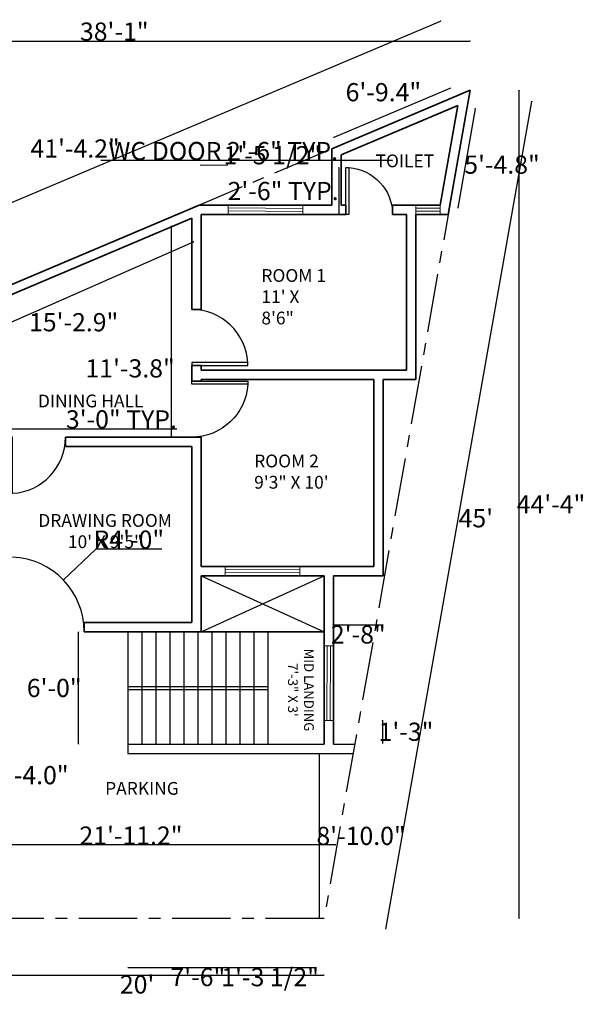
# Model space of a CAD drawing. Units: inches. Extents: x -496 to 183, y 146 to 778.
# Tile 2 of 2: x -180 to 183, y 146 to 778. Entities that reach past the tile are written whole.
import ezdxf

# ---------------------------------------------------------------- set-up
doc = ezdxf.new("R2010")
doc.units = ezdxf.units.IN
doc.header["$MEASUREMENT"] = 0
doc.linetypes.add('CENTER', pattern=[2, 1.25, -0.25, 0.25, -0.25])
for name, color, linetype, lineweight in [('A-ANNO-DIMS', 5, 'Continuous', 18), ('A-AREA-IDEN', 7, 'Continuous', 18), ('A-DOOR', 30, 'Continuous', 25), ('A-FLOR-STRS', 7, 'Continuous', 25), ('A-GLAZ', 2, 'Continuous', 18), ('A-WALL', 7, 'Continuous', 35), ('C-PROP', 3, 'CENTER', 25)]:
    doc.layers.add(name, color=color, linetype=linetype, lineweight=lineweight)
doc.styles.get("Standard").update_dxf_attribs({"font": 'arial.ttf'})
doc.dimstyles.get("Standard").update_dxf_attribs({"dimtxt": 11.68, "dimasz": 0.18, "dimexe": 0.18, "dimexo": 0.0625, "dimgap": 0.09, "dimtad": 2, "dimtih": 1, "dimtoh": 1, "dimdec": 1, "dimzin": 0, "dimdsep": 46, "dimlunit": 3, "dimtxsty": 'Standard', "dimblk": 'OPEN30', "dimcen": 0.09, "dimse1": 1, "dimse2": 1, "dimadec": 0, "dimazin": 0, "dimtfac": 1, "dimtdec": 1, "dimtofl": 0, "dimtmove": 0, "dimatfit": 3, "dimfxl": 1, "dimtolj": 1, "dimtzin": 0, "dimarcsym": 0})

# ---------------------------------------------------------------- blocks, each defined once
blk = doc.blocks.new('_Open30')
at = {"color": 0, "linetype": 'ByBlock', "lineweight": -2}
for p, q in [((-1, 0.27), (0, 0)), ((0, 0), (-1, -0.27)), ((0, 0), (-1, 0))]:
    blk.add_line(p, q, dxfattribs=at)
blk = doc.blocks.new('*D3')
at = {"layer": 'A-ANNO-DIMS', "color": 0, "lineweight": -2, "ltscale": 5, "transparency": 16777216}
blk.add_line((-224.62, 164.47), (15.02, 164.47), dxfattribs=at)
at = {"layer": 'Defpoints', "color": 0, "ltscale": 5, "transparency": 16777216}
for p in [(-224.8, 200.81), (15.2, 200.81), (15.2, 164.47)]:
    blk.add_point(p, dxfattribs=at)
at = {"layer": 'A-ANNO-DIMS', "color": 0, "lineweight": -2, "ltscale": 5, "transparency": 16777216, "xscale": 0.18, "yscale": 0.18, "zscale": 0.18, "rotation": 180}
blk.add_blockref('_Open30', (-224.8, 164.47), dxfattribs=at)
at = {"layer": 'A-ANNO-DIMS', "color": 0, "lineweight": -2, "ltscale": 5, "transparency": 16777216, "xscale": 0.18, "yscale": 0.18, "zscale": 0.18}
blk.add_blockref('_Open30', (15.2, 164.47), dxfattribs=at)
at = {"layer": 'A-ANNO-DIMS', "color": 0, "ltscale": 5, "transparency": 16777216, "insert": (-104.8, 158.42), "char_height": 11.68, "attachment_point": 5}
blk.add_mtext("\\A1;20'", dxfattribs=at)
blk = doc.blocks.new('*D4')
at = {"layer": 'A-ANNO-DIMS', "color": 0, "lineweight": -2, "ltscale": 5, "transparency": 16777216}
blk.add_line((54.9, 194), (148.6, 725.44), dxfattribs=at)
at = {"layer": 'Defpoints', "color": 0, "ltscale": 5, "transparency": 16777216}
for p in [(108.97, 732.61), (148.63, 725.62), (15.2, 200.81)]:
    blk.add_point(p, dxfattribs=at)
at = {"layer": 'A-ANNO-DIMS', "color": 0, "lineweight": -2, "ltscale": 5, "transparency": 16777216, "xscale": 0.18, "yscale": 0.18, "zscale": 0.18}
for p, rotation in [((148.63, 725.62), 80), ((54.86, 193.82), 260)]:
    blk.add_blockref('_Open30', p, dxfattribs=dict(at, rotation=rotation))
at = {"layer": 'A-ANNO-DIMS', "color": 0, "ltscale": 5, "transparency": 16777216, "insert": (112.71, 457.79), "char_height": 11.68, "attachment_point": 5}
blk.add_mtext("\\A1;45'", dxfattribs=at)
blk = doc.blocks.new('*D6')
at = {"layer": 'A-ANNO-DIMS', "color": 0, "lineweight": -2, "ltscale": 5, "transparency": 16777216}
blk.add_line((-366.62, 583.72), (89.94, 777.08), dxfattribs=at)
at = {"layer": 'Defpoints', "color": 0, "ltscale": 5, "transparency": 16777216}
for p in [(90.11, 777.15), (108.97, 732.61), (-347.92, 539.1)]:
    blk.add_point(p, dxfattribs=at)
at = {"layer": 'A-ANNO-DIMS', "color": 0, "lineweight": -2, "ltscale": 5, "transparency": 16777216, "xscale": 0.18, "yscale": 0.18, "zscale": 0.18}
for p, rotation in [((90.11, 777.15), 22.95381137769926), ((-366.79, 583.64), 202.9538113776993)]:
    blk.add_blockref('_Open30', p, dxfattribs=dict(at, rotation=rotation))
at = {"layer": 'A-ANNO-DIMS', "color": 0, "ltscale": 5, "transparency": 16777216, "insert": (-144.61, 695.21), "char_height": 11.68, "attachment_point": 5}
blk.add_mtext('\\A1;41\'-4.2"', dxfattribs=at)
blk = doc.blocks.new('*D7')
at = {"layer": 'A-ANNO-DIMS', "color": 0, "lineweight": -2, "ltscale": 5, "transparency": 16777216}
blk.add_line((-235.59, 561.64), (-68.58, 635.31), dxfattribs=at)
at = {"layer": 'Defpoints', "color": 0, "ltscale": 5, "transparency": 16777216}
for p in [(-69.77, 638.45), (-68.41, 635.38), (-237.11, 564.64)]:
    blk.add_point(p, dxfattribs=at)
at = {"layer": 'A-ANNO-DIMS', "color": 0, "lineweight": -2, "ltscale": 5, "transparency": 16777216, "xscale": 0.18, "yscale": 0.18, "zscale": 0.18}
for p, rotation in [((-68.41, 635.38), 23.80147962325558), ((-235.75, 561.57), 203.8014796232556)]:
    blk.add_blockref('_Open30', p, dxfattribs=dict(at, rotation=rotation))
at = {"layer": 'A-ANNO-DIMS', "color": 0, "ltscale": 5, "transparency": 16777216, "insert": (-145.55, 583.66), "char_height": 11.68, "attachment_point": 5}
blk.add_mtext('\\A1;15\'-2.9"', dxfattribs=at)
blk = doc.blocks.new('*D8')
at = {"layer": 'A-ANNO-DIMS', "color": 0, "lineweight": -2, "ltscale": 5, "transparency": 16777216}
blk.add_line((-82.89, 645.46), (-82.89, 509.99), dxfattribs=at)
at = {"layer": 'Defpoints', "color": 0, "ltscale": 5, "transparency": 16777216}
for p in [(-80.99, 645.64), (-82.89, 509.81), (-80.99, 509.81)]:
    blk.add_point(p, dxfattribs=at)
at = {"layer": 'A-ANNO-DIMS', "color": 0, "lineweight": -2, "ltscale": 5, "transparency": 16777216, "xscale": 0.18, "yscale": 0.18, "zscale": 0.18}
for p, rotation in [((-82.89, 645.64), 90), ((-82.89, 509.81), 270)]:
    blk.add_blockref('_Open30', p, dxfattribs=dict(at, rotation=rotation))
at = {"layer": 'A-ANNO-DIMS', "color": 0, "ltscale": 5, "transparency": 16777216, "insert": (-109.3, 554.01), "char_height": 11.68, "attachment_point": 5}
blk.add_mtext('\\A1;11\'-3.8"', dxfattribs=at)
blk = doc.blocks.new('*D9')
at = {"layer": 'A-ANNO-DIMS', "color": 0, "lineweight": -2, "ltscale": 5, "transparency": 16777216}
blk.add_line((112.33, 720.62), (101.13, 657.13), dxfattribs=at)
at = {"layer": 'Defpoints', "color": 0, "ltscale": 5, "transparency": 16777216}
for p in [(101.15, 722.78), (89.89, 658.93), (101.1, 656.96)]:
    blk.add_point(p, dxfattribs=at)
at = {"layer": 'A-ANNO-DIMS', "color": 0, "lineweight": -2, "ltscale": 5, "transparency": 16777216, "xscale": 0.18, "yscale": 0.18, "zscale": 0.18}
for p, rotation in [((112.36, 720.8), 79.99999999999996), ((101.1, 656.96), 260)]:
    blk.add_blockref('_Open30', p, dxfattribs=dict(at, rotation=rotation))
at = {"layer": 'A-ANNO-DIMS', "color": 0, "ltscale": 5, "transparency": 16777216, "insert": (129.51, 684.86), "char_height": 11.68, "attachment_point": 5}
blk.add_mtext('\\A1;5\'-4.8"', dxfattribs=at)
blk = doc.blocks.new('*D10')
at = {"layer": 'A-ANNO-DIMS', "color": 0, "lineweight": -2, "ltscale": 5, "transparency": 16777216}
blk.add_line((21.63, 702.39), (96.21, 733.98), dxfattribs=at)
at = {"layer": 'Defpoints', "color": 0, "ltscale": 5, "transparency": 16777216}
for p in [(96.37, 734.05), (101.15, 722.78), (26.23, 691.05)]:
    blk.add_point(p, dxfattribs=at)
at = {"layer": 'A-ANNO-DIMS', "color": 0, "lineweight": -2, "ltscale": 5, "transparency": 16777216, "xscale": 0.18, "yscale": 0.18, "zscale": 0.18}
for p, rotation in [((96.37, 734.05), 22.95381137769932), ((21.46, 702.32), 202.9538113776993)]:
    blk.add_blockref('_Open30', p, dxfattribs=dict(at, rotation=rotation))
at = {"layer": 'A-ANNO-DIMS', "color": 0, "ltscale": 5, "transparency": 16777216, "insert": (53.33, 731.38), "char_height": 11.68, "attachment_point": 5}
blk.add_mtext('\\A1;6\'-9.4"', dxfattribs=at)
blk = doc.blocks.new('*D11')
at = {"layer": 'A-ANNO-DIMS', "color": 0, "lineweight": -2, "ltscale": 5, "transparency": 16777216}
blk.add_line((12.02, 306.63), (12.02, 200.99), dxfattribs=at)
at = {"layer": 'Defpoints', "color": 0, "ltscale": 5, "transparency": 16777216}
for p in [(4.85, 306.81), (4.85, 200.81), (12.02, 200.81)]:
    blk.add_point(p, dxfattribs=at)
at = {"layer": 'A-ANNO-DIMS', "color": 0, "lineweight": -2, "ltscale": 5, "transparency": 16777216, "xscale": 0.18, "yscale": 0.18, "zscale": 0.18}
for p, rotation in [((12.02, 306.81), 90), ((12.02, 200.81), 270)]:
    blk.add_blockref('_Open30', p, dxfattribs=dict(at, rotation=rotation))
at = {"layer": 'A-ANNO-DIMS', "color": 0, "ltscale": 5, "transparency": 16777216, "insert": (38.99, 253.81), "char_height": 11.68, "attachment_point": 5}
blk.add_mtext('\\A1;8\'-10.0"', dxfattribs=at)
blk = doc.blocks.new('*D12')
at = {"layer": 'A-ANNO-DIMS', "color": 0, "lineweight": -2, "ltscale": 5, "transparency": 16777216}
blk.add_line((22.65, 248.06), (-240.18, 248.06), dxfattribs=at)
at = {"layer": 'Defpoints', "color": 0, "ltscale": 5, "transparency": 16777216}
for p in [(-240.36, 248.06), (-240.36, 243.58), (22.83, 244.08)]:
    blk.add_point(p, dxfattribs=at)
at = {"layer": 'A-ANNO-DIMS', "color": 0, "lineweight": -2, "ltscale": 5, "transparency": 16777216, "xscale": 0.18, "yscale": 0.18, "zscale": 0.18, "rotation": 180}
blk.add_blockref('_Open30', (-240.36, 248.06), dxfattribs=at)
at = {"layer": 'A-ANNO-DIMS', "color": 0, "lineweight": -2, "ltscale": 5, "transparency": 16777216, "xscale": 0.18, "yscale": 0.18, "zscale": 0.18}
blk.add_blockref('_Open30', (22.83, 248.06), dxfattribs=at)
at = {"layer": 'A-ANNO-DIMS', "color": 0, "ltscale": 5, "transparency": 16777216, "insert": (-108.76, 254.01), "char_height": 11.68, "attachment_point": 5}
blk.add_mtext('\\A1;21\'-11.2"', dxfattribs=at)
blk = doc.blocks.new('*D13')
at = {"layer": 'A-ANNO-DIMS', "color": 0, "lineweight": -2, "ltscale": 5, "transparency": 16777216}
blk.add_line((-203.87, 200.99), (-203.87, 384.63), dxfattribs=at)
at = {"layer": 'Defpoints', "color": 0, "ltscale": 5, "transparency": 16777216}
for p in [(-208.53, 384.81), (-203.87, 384.81), (-208.53, 200.81)]:
    blk.add_point(p, dxfattribs=at)
at = {"layer": 'A-ANNO-DIMS', "color": 0, "lineweight": -2, "ltscale": 5, "transparency": 16777216, "xscale": 0.18, "yscale": 0.18, "zscale": 0.18}
for p, rotation in [((-203.87, 384.81), 90), ((-203.87, 200.81), 270)]:
    blk.add_blockref('_Open30', p, dxfattribs=dict(at, rotation=rotation))
at = {"layer": 'A-ANNO-DIMS', "color": 0, "ltscale": 5, "transparency": 16777216, "insert": (-177.47, 292.81), "char_height": 11.68, "attachment_point": 5}
blk.add_mtext('\\A1;15\'-4.0"', dxfattribs=at)
blk = doc.blocks.new('DOOR-SWING-36IN')
at = {"ltscale": 5}
for p, q in [((0, 0), (0, -36)), ((2, 0), (0, 0)), ((2, -36), (2, 0)), ((0, -36), (2, -36))]:
    blk.add_line(p, q, dxfattribs=at)
blk.add_arc((-0.06, 0), 36.06, 273.27315, 0, dxfattribs=at)
blk = doc.blocks.new('DOOR-SWING-30IN')
at = {"ltscale": 5}
for p, q in [((0, 0), (-30, 0)), ((-30, 0), (-30, -2)), ((0, -2), (0, 0)), ((-30, -2), (0, -2))]:
    blk.add_line(p, q, dxfattribs=at)
blk.add_arc((0, 0.07), 30.07, 183.94987, 270, dxfattribs=at)
blk = doc.blocks.new('WIN-48IN')
at = {"ltscale": 5}
for p, q in [((0, 0), (-0.22, -48)), ((0, 0), (6, -0.03)), ((6, -0.03), (5.78, -48.03)), ((-0.22, -48), (5.78, -48.03))]:
    blk.add_line(p, q, dxfattribs=at)
for p, q in [((1.78, -48.01), (2, -0.01)), ((3.78, -48.02), (4, -0.02))]:
    blk.add_line(p, q)
blk = doc.blocks.new('WIN-SMALL-WC')
at = {"ltscale": 5}
for p, q in [((-15.66, -6), (-15.66, 0)), ((-15.66, 0), (0, 0)), ((0, 0), (0, -6)), ((-15.66, -2), (0, -2)), ((0, -4), (-15.66, -4)), ((0, -6), (-15.66, -6))]:
    blk.add_line(p, q, dxfattribs=at)
blk = doc.blocks.new('*D21')
at = {"layer": 'A-ANNO-DIMS', "color": 0, "lineweight": -2, "ltscale": 5, "transparency": 16777216}
for p, q in [((-186.59, 515.21), (-150.95, 515.21)), ((-150.77, 515.21), (-79.22, 515.21))]:
    blk.add_line(p, q, dxfattribs=at)
at = {"layer": 'Defpoints', "color": 0, "ltscale": 5, "transparency": 16777216}
for p in [(-150.77, 515.21), (-186.77, 509.81), (-150.77, 509.81)]:
    blk.add_point(p, dxfattribs=at)
at = {"layer": 'A-ANNO-DIMS', "color": 0, "lineweight": -2, "ltscale": 5, "transparency": 16777216, "xscale": 0.18, "yscale": 0.18, "zscale": 0.18, "rotation": 180}
blk.add_blockref('_Open30', (-186.77, 515.21), dxfattribs=at)
at = {"layer": 'A-ANNO-DIMS', "color": 0, "lineweight": -2, "ltscale": 5, "transparency": 16777216, "xscale": 0.18, "yscale": 0.18, "zscale": 0.18}
blk.add_blockref('_Open30', (-150.77, 515.21), dxfattribs=at)
at = {"layer": 'A-ANNO-DIMS', "color": 0, "ltscale": 5, "transparency": 16777216, "insert": (-114.9, 521.27), "char_height": 11.68, "attachment_point": 5}
blk.add_mtext('\\A1;3\'-0" TYP.', dxfattribs=at)
blk = doc.blocks.new('*D22')
at = {"layer": 'A-ANNO-DIMS', "color": 0, "lineweight": -2, "ltscale": 5, "transparency": 16777216}
for p, q in [((29.23, 687.43), (-128, 687.43)), ((59.05, 687.43), (29.41, 687.43))]:
    blk.add_line(p, q, dxfattribs=at)
at = {"layer": 'Defpoints', "color": 0, "ltscale": 5, "transparency": 16777216}
for p in [(29.23, 687.43), (29.23, 682.93), (59.23, 682.93)]:
    blk.add_point(p, dxfattribs=at)
at = {"layer": 'A-ANNO-DIMS', "color": 0, "lineweight": -2, "ltscale": 5, "transparency": 16777216, "xscale": 0.18, "yscale": 0.18, "zscale": 0.18}
for p, rotation in [((29.23, 687.43), 179.9999999999994), ((59.23, 687.43), 359.9999999999994)]:
    blk.add_blockref('_Open30', p, dxfattribs=dict(at, rotation=rotation))
at = {"layer": 'A-ANNO-DIMS', "color": 0, "ltscale": 5, "transparency": 16777216, "insert": (-49.47, 693.57), "char_height": 11.68, "attachment_point": 5}
blk.add_mtext('\\A1;WC DOOR 2\'-6" TYP.', dxfattribs=at)
blk = doc.blocks.new('*D23')
at = {"layer": 'A-ANNO-DIMS', "color": 0, "lineweight": -2, "ltscale": 5, "transparency": 16777216}
blk.add_line((24.73, 682.75), (24.73, 653.11), dxfattribs=at)
at = {"layer": 'Defpoints', "color": 0, "ltscale": 5, "transparency": 16777216}
for p in [(29.23, 682.93), (24.73, 652.93), (29.23, 652.93)]:
    blk.add_point(p, dxfattribs=at)
at = {"layer": 'A-ANNO-DIMS', "color": 0, "lineweight": -2, "ltscale": 5, "transparency": 16777216, "xscale": 0.18, "yscale": 0.18, "zscale": 0.18}
for p, rotation in [((24.73, 682.93), 90), ((24.73, 652.93), 270)]:
    blk.add_blockref('_Open30', p, dxfattribs=dict(at, rotation=rotation))
at = {"layer": 'A-ANNO-DIMS', "color": 0, "ltscale": 5, "transparency": 16777216, "insert": (-11.05, 667.93), "char_height": 11.68, "attachment_point": 5}
blk.add_mtext('\\A1;2\'-6" TYP.', dxfattribs=at)
blk = doc.blocks.new('*D28')
at = {"layer": 'A-ANNO-DIMS', "color": 0, "lineweight": -2, "ltscale": 5, "transparency": 16777216}
blk.add_line((-347.74, 764.21), (108.79, 764.21), dxfattribs=at)
at = {"layer": 'Defpoints', "color": 0, "ltscale": 5, "transparency": 16777216}
for p in [(108.97, 764.21), (108.97, 732.61), (-347.92, 539.1)]:
    blk.add_point(p, dxfattribs=at)
at = {"layer": 'A-ANNO-DIMS', "color": 0, "lineweight": -2, "ltscale": 5, "transparency": 16777216, "xscale": 0.18, "yscale": 0.18, "zscale": 0.18, "rotation": 180}
blk.add_blockref('_Open30', (-347.92, 764.21), dxfattribs=at)
at = {"layer": 'A-ANNO-DIMS', "color": 0, "lineweight": -2, "ltscale": 5, "transparency": 16777216, "xscale": 0.18, "yscale": 0.18, "zscale": 0.18}
blk.add_blockref('_Open30', (108.97, 764.21), dxfattribs=at)
at = {"layer": 'A-ANNO-DIMS', "color": 0, "ltscale": 5, "transparency": 16777216, "insert": (-119.47, 770.27), "char_height": 11.68, "attachment_point": 5}
blk.add_mtext('\\A1;38\'-1"', dxfattribs=at)
blk = doc.blocks.new('*D29')
at = {"layer": 'A-ANNO-DIMS', "color": 0, "lineweight": -2, "ltscale": 5, "transparency": 16777216}
blk.add_line((140.57, 200.99), (140.57, 732.43), dxfattribs=at)
at = {"layer": 'Defpoints', "color": 0, "ltscale": 5, "transparency": 16777216}
for p in [(108.97, 732.61), (140.57, 732.61), (15.2, 200.81)]:
    blk.add_point(p, dxfattribs=at)
at = {"layer": 'A-ANNO-DIMS', "color": 0, "lineweight": -2, "ltscale": 5, "transparency": 16777216, "xscale": 0.18, "yscale": 0.18, "zscale": 0.18}
for p, rotation in [((140.57, 732.61), 90), ((140.57, 200.81), 270)]:
    blk.add_blockref('_Open30', p, dxfattribs=dict(at, rotation=rotation))
at = {"layer": 'A-ANNO-DIMS', "color": 0, "ltscale": 5, "transparency": 16777216, "insert": (160.96, 466.71), "char_height": 11.68, "attachment_point": 5}
blk.add_mtext('\\A1;44\'-4"', dxfattribs=at)
blk = doc.blocks.new('*D30')
at = {"layer": 'A-ANNO-DIMS', "color": 0, "lineweight": -2, "ltscale": 5, "transparency": 16777216}
blk.add_line((-110.62, 169.21), (-20.98, 169.21), dxfattribs=at)
at = {"layer": 'Defpoints', "color": 0, "ltscale": 5, "transparency": 16777216}
for p in [(-110.8, 312.81), (-20.8, 312.81), (-20.8, 169.21)]:
    blk.add_point(p, dxfattribs=at)
at = {"layer": 'A-ANNO-DIMS', "color": 0, "lineweight": -2, "ltscale": 5, "transparency": 16777216, "xscale": 0.18, "yscale": 0.18, "zscale": 0.18, "rotation": 180}
blk.add_blockref('_Open30', (-110.8, 169.21), dxfattribs=at)
at = {"layer": 'A-ANNO-DIMS', "color": 0, "lineweight": -2, "ltscale": 5, "transparency": 16777216, "xscale": 0.18, "yscale": 0.18, "zscale": 0.18}
blk.add_blockref('_Open30', (-20.8, 169.21), dxfattribs=at)
at = {"layer": 'A-ANNO-DIMS', "color": 0, "ltscale": 5, "transparency": 16777216, "insert": (-65.8, 163.16), "char_height": 11.68, "attachment_point": 5}
blk.add_mtext('\\A1;7\'-6"', dxfattribs=at)
blk = doc.blocks.new('*D33')
at = {"layer": 'A-ANNO-DIMS', "color": 0, "lineweight": -2, "ltscale": 5, "transparency": 16777216}
for p, q in [((-63.59, 169.21), (-48.43, 169.21)), ((-48.25, 169.21), (9.27, 169.21))]:
    blk.add_line(p, q, dxfattribs=at)
at = {"layer": 'Defpoints', "color": 0, "ltscale": 5, "transparency": 16777216}
for p in [(-63.77, 426.81), (-48.25, 426.92), (-48.25, 169.21)]:
    blk.add_point(p, dxfattribs=at)
at = {"layer": 'A-ANNO-DIMS', "color": 0, "lineweight": -2, "ltscale": 5, "transparency": 16777216, "xscale": 0.18, "yscale": 0.18, "zscale": 0.18, "rotation": 180}
blk.add_blockref('_Open30', (-63.77, 169.21), dxfattribs=at)
at = {"layer": 'A-ANNO-DIMS', "color": 0, "lineweight": -2, "ltscale": 5, "transparency": 16777216, "xscale": 0.18, "yscale": 0.18, "zscale": 0.18}
blk.add_blockref('_Open30', (-48.25, 169.21), dxfattribs=at)
at = {"layer": 'A-ANNO-DIMS', "color": 0, "ltscale": 5, "transparency": 16777216, "insert": (-19.4, 163.08), "char_height": 11.68, "attachment_point": 5}
blk.add_mtext('\\A1;1\'-3 1/2"', dxfattribs=at)
blk = doc.blocks.new('*D34')
at = {"layer": 'A-ANNO-DIMS', "color": 0, "lineweight": -2, "ltscale": 5, "transparency": 16777216}
for p, q in [((-63.98, 684.53), (-47, 684.74)), ((-46.82, 684.75), (-46.64, 684.75))]:
    blk.add_line(p, q, dxfattribs=at)
at = {"layer": 'Defpoints', "color": 0, "ltscale": 5, "transparency": 16777216}
for p in [(-46.82, 684.75), (-63.77, 652.93), (-46.43, 653.15)]:
    blk.add_point(p, dxfattribs=at)
at = {"layer": 'A-ANNO-DIMS', "color": 0, "lineweight": -2, "ltscale": 5, "transparency": 16777216, "xscale": 0.18, "yscale": 0.18, "zscale": 0.18}
for p, rotation in [((-64.16, 684.53), 180.7141226270407), ((-46.82, 684.75), 0.7141226270407911)]:
    blk.add_blockref('_Open30', p, dxfattribs=dict(at, rotation=rotation))
at = {"layer": 'A-ANNO-DIMS', "color": 0, "ltscale": 5, "transparency": 16777216, "insert": (-17.97, 690.88), "char_height": 11.68, "attachment_point": 5}
blk.add_mtext('\\A1;1\'-5 1/2"', dxfattribs=at)
blk = doc.blocks.new('*D36')
at = {"layer": 'A-ANNO-DIMS', "color": 0, "lineweight": -2, "ltscale": 5, "transparency": 16777216}
blk.add_line((53.05, 389.21), (21.38, 389.21), dxfattribs=at)
at = {"layer": 'Defpoints', "color": 0, "ltscale": 5, "transparency": 16777216}
for p in [(21.2, 420.81), (53.23, 420.81), (21.2, 389.21)]:
    blk.add_point(p, dxfattribs=at)
at = {"layer": 'A-ANNO-DIMS', "color": 0, "lineweight": -2, "ltscale": 5, "transparency": 16777216, "xscale": 0.18, "yscale": 0.18, "zscale": 0.18, "rotation": 180}
blk.add_blockref('_Open30', (21.2, 389.21), dxfattribs=at)
at = {"layer": 'A-ANNO-DIMS', "color": 0, "lineweight": -2, "ltscale": 5, "transparency": 16777216, "xscale": 0.18, "yscale": 0.18, "zscale": 0.18}
blk.add_blockref('_Open30', (53.23, 389.21), dxfattribs=at)
at = {"layer": 'A-ANNO-DIMS', "color": 0, "ltscale": 5, "transparency": 16777216, "insert": (37.22, 383.16), "char_height": 11.68, "attachment_point": 5}
blk.add_mtext('\\A1;2\'-8"', dxfattribs=at)
blk = doc.blocks.new('*D37')
at = {"layer": 'A-ANNO-DIMS', "color": 0, "lineweight": -2, "ltscale": 5, "transparency": 16777216}
blk.add_line((-142.4, 312.99), (-142.4, 384.63), dxfattribs=at)
at = {"layer": 'Defpoints', "color": 0, "ltscale": 5, "transparency": 16777216}
for p in [(-142.4, 384.81), (-110.8, 384.81), (-110.8, 312.81)]:
    blk.add_point(p, dxfattribs=at)
at = {"layer": 'A-ANNO-DIMS', "color": 0, "lineweight": -2, "ltscale": 5, "transparency": 16777216, "xscale": 0.18, "yscale": 0.18, "zscale": 0.18}
for p, rotation in [((-142.4, 384.81), 90), ((-142.4, 312.81), 270)]:
    blk.add_blockref('_Open30', p, dxfattribs=dict(at, rotation=rotation))
at = {"layer": 'A-ANNO-DIMS', "color": 0, "ltscale": 5, "transparency": 16777216, "insert": (-158.04, 348.81), "char_height": 11.68, "attachment_point": 5}
blk.add_mtext('\\A1;6\'-0"', dxfattribs=at)
blk = doc.blocks.new('*D38')
at = {"layer": 'A-ANNO-DIMS', "color": 0, "lineweight": -2, "ltscale": 5, "transparency": 16777216}
blk.add_line((52.7, 327.95), (52.8, 313.22), dxfattribs=at)
at = {"layer": 'Defpoints', "color": 0, "ltscale": 5, "transparency": 16777216}
for p in [(21.1, 327.9), (21.2, 312.81), (52.8, 313.04)]:
    blk.add_point(p, dxfattribs=at)
at = {"layer": 'A-ANNO-DIMS', "color": 0, "lineweight": -2, "ltscale": 5, "transparency": 16777216, "xscale": 0.18, "yscale": 0.18, "zscale": 0.18}
for p, rotation in [((52.7, 328.13), 90.41009353427447), ((52.8, 313.04), 270.4100935342744)]:
    blk.add_blockref('_Open30', p, dxfattribs=dict(at, rotation=rotation))
at = {"layer": 'A-ANNO-DIMS', "color": 0, "ltscale": 5, "transparency": 16777216, "insert": (67.86, 320.69), "char_height": 11.68, "attachment_point": 5}
blk.add_mtext('\\A1;1\'-3"', dxfattribs=at)
blk = doc.blocks.new('*D40')
at = {"layer": 'A-ANNO-DIMS', "color": 0, "lineweight": -2, "ltscale": 5, "transparency": 16777216}
for p, q in [((-131.31, 438), (-151.99, 418.18)), ((-88.99, 438), (-131.31, 438)), ((-186.9, 384.81), (-186.72, 384.81)), ((-186.81, 384.72), (-186.81, 384.9))]:
    blk.add_line(p, q, dxfattribs=at)
at = {"layer": 'Defpoints', "color": 0, "ltscale": 5, "transparency": 16777216}
for p in [(-152.12, 418.05), (-186.81, 384.81)]:
    blk.add_point(p, dxfattribs=at)
at = {"layer": 'A-ANNO-DIMS', "color": 0, "lineweight": -2, "ltscale": 5, "transparency": 16777216, "xscale": 0.18, "yscale": 0.18, "zscale": 0.18, "rotation": 223.7807826130634}
blk.add_blockref('_Open30', (-152.12, 418.05), dxfattribs=at)
at = {"layer": 'A-ANNO-DIMS', "color": 0, "ltscale": 5, "transparency": 16777216, "insert": (-110.11, 444.05), "char_height": 11.68, "attachment_point": 5}
blk.add_mtext('\\A1;R4\'-0"', dxfattribs=at)

msp = doc.modelspace()

# ---------------------------------------------------------------- linework, layer by layer
at = {"layer": 'A-DOOR', "ltscale": 5}
msp.add_arc((-186.81, 384.81), 48.04, 0, 87.56225, dxfattribs=at)
at = {"layer": 'A-FLOR-STRS'}
for p, q in [((-63.77, 384.81), (15.2, 420.81)), ((-63.77, 420.81), (15.2, 384.81)), ((-110.8, 384.81), (-110.8, 306.81)), ((-101.8, 384.81), (-101.8, 312.81)), ((-92.8, 384.81), (-92.8, 312.81)), ((-83.8, 384.81), (-83.8, 312.81)), ((-74.8, 384.81), (-74.8, 312.81)), ((-65.8, 384.81), (-65.8, 312.81)), ((-56.8, 384.81), (-56.8, 312.81)), ((-47.8, 384.81), (-47.8, 312.81)), ((-38.8, 384.81), (-38.8, 312.81)), ((-29.8, 384.81), (-29.8, 312.81)), ((-20.8, 384.81), (-20.8, 312.81)), ((-110.8, 349.81), (-20.8, 349.81)), ((-110.8, 347.81), (-20.8, 347.81)), ((-110.8, 312.81), (15.2, 312.81)), ((21.2, 312.81), (34.95, 312.81)), ((-110.8, 306.81), (33.9, 306.81))]:
    msp.add_line(p, q, dxfattribs=at)
at = {"layer": 'A-WALL', "ltscale": 5}
for p, q in [((20.23, 695.02), (108.97, 732.61)), ((108.97, 732.61), (94.93, 652.93)), ((-64.98, 658.93), (-325.77, 548.48))]:
    msp.add_line(p, q, dxfattribs=at)
at = {"layer": 'A-WALL'}
for p, q in [((101.15, 722.78), (26.23, 691.05)), ((89.89, 658.93), (101.15, 722.78)), ((20.23, 658.93), (20.23, 695.02)), ((26.23, 658.93), (26.23, 691.05)), ((-64.98, 658.93), (20.23, 658.93)), ((26.23, 658.93), (29.23, 658.93)), ((29.23, 652.93), (29.23, 658.93)), ((59.23, 652.93), (59.23, 658.93)), ((59.23, 658.93), (89.89, 658.93)), ((-63.77, 652.93), (29.23, 652.93)), ((-63.77, 591.81), (-63.77, 652.93)), ((59.23, 652.93), (68.23, 652.93)), ((68.23, 552.81), (68.23, 652.93)), ((74.23, 546.81), (74.23, 652.93)), ((74.23, 652.93), (94.93, 652.93)), ((-69.77, 650.39), (-319.79, 544.5)), ((-69.77, 591.81), (-69.77, 650.39)), ((-69.77, 591.81), (-63.77, 591.81)), ((-69.77, 545.81), (-69.77, 555.81)), ((-69.77, 555.81), (-63.77, 555.81)), ((-63.77, 552.81), (-63.77, 555.81)), ((-63.77, 552.81), (68.23, 552.81)), ((-69.77, 545.81), (-63.77, 545.81)), ((-63.77, 545.81), (-63.77, 546.81)), ((-63.77, 546.81), (47.23, 546.81)), ((47.23, 426.81), (47.23, 546.81)), ((53.23, 420.81), (53.23, 546.81)), ((53.23, 546.81), (74.23, 546.81)), ((-150.77, 503.81), (-150.77, 509.81)), ((-150.77, 509.81), (-63.77, 509.81)), ((-63.77, 426.81), (-63.77, 509.81)), ((-150.77, 503.81), (-69.77, 503.81)), ((-69.77, 390.81), (-69.77, 503.81)), ((-63.77, 426.81), (47.23, 426.81)), ((-63.77, 384.81), (-63.77, 420.81)), ((-63.77, 420.81), (15.2, 420.81)), ((15.2, 420.81), (15.2, 312.81)), ((21.2, 420.81), (53.23, 420.81)), ((21.2, 420.81), (21.2, 312.81)), ((-138.77, 384.81), (-138.77, 390.81)), ((-138.77, 390.81), (-69.77, 390.81)), ((-138.77, 384.81), (15.2, 384.81))]:
    msp.add_line(p, q, dxfattribs=at)
at = {"layer": 'C-PROP', "ltscale": 30}
msp.add_lwpolyline([(-320.16, 462.81), (-347.92, 539.1), (108.97, 732.61), (15.2, 200.81), (-224.8, 200.81), (-319.06, 459.81)], close=True, dxfattribs=at)

# ---------------------------------------------------------------- block references
at = {"layer": 'A-DOOR', "extrusion": (0, 0, -1), "zscale": -1}
for name, p, rotation in [('DOOR-SWING-30IN', (-29.23, 652.93), 270.0000000000006), ('DOOR-SWING-36IN', (69.77, 545.81), 270.0000000000001)]:
    msp.add_blockref(name, p, dxfattribs=dict(at, rotation=rotation))
at = {"layer": 'A-DOOR', "rotation": 90.0000000000006}
msp.add_blockref('DOOR-SWING-36IN', (-69.77, 555.81), dxfattribs=at)
at = {"layer": 'A-DOOR'}
msp.add_blockref('DOOR-SWING-36IN', (-186.77, 509.81), dxfattribs=at)
at = {"layer": 'A-GLAZ'}
for p, rotation in [((1.62, 658.72), 269.7423272106765), ((-48.28, 420.92), 90.00000000000017), ((21.1, 327.9), 180)]:
    msp.add_blockref('WIN-48IN', p, dxfattribs=dict(at, rotation=rotation))
msp.add_blockref('WIN-SMALL-WC', (89.89, 658.93), dxfattribs=at)

# ---------------------------------------------------------------- texts
at = {"layer": 'A-AREA-IDEN', "ltscale": 5, "char_height": 8.2, "attachment_point": 1}
for s, width, insert in [('TOILET', 1.3024, (48.29, 691.38)), ('ROOM 1\\P11\' X 8\'6"', 47.3032, (-25.02, 617.79)), ('DINING HALL', 75.8236, (-168.49, 537.2)), ('ROOM 2\\P9\'3" X 10\'', 48.5564, (-29.63, 498.65)), ('\\pxqc;DRAWING ROOM\\P10\' X 9\'5"', 94.5703, (-172.65, 460.47)), ('PARKING', 1.3024, (-125.34, 288.43))]:
    msp.add_mtext_dynamic_manual_height_columns(s, width=width, gutter_width=1, heights=[0], dxfattribs=dict(at, insert=insert))
at = {"layer": 'A-AREA-IDEN', "ltscale": 5, "insert": (8.64, 384.81), "char_height": 6.2, "attachment_point": 1, "rotation": 270}
msp.add_mtext_dynamic_manual_height_columns('\\pxqc;MID LANDING\\P7\'-3" X 3\'', width=74.5449, gutter_width=1, heights=[0], dxfattribs=at)

# ---------------------------------------------------------------- dimensions: what is measured, and where the dimension line sits
at = {"layer": 'A-ANNO-DIMS', "ltscale": 5}
for base, p1, p2, override, picture, middle in [((108.97, 764.21), (-347.92, 539.1), (108.97, 732.61), {"dimdec": 1, "dimlfac": 1, "dimrnd": 0, "dimzin": 1, "dimdsep": 46, "dimlunit": 4, "dimfrac": 2}, '*D28', (-119.47, 770.27)), ((-48.25, 169.21), (-63.77, 426.81), (-48.25, 426.92), {"dimdec": 1, "dimlfac": 1, "dimrnd": 0, "dimzin": 1, "dimdsep": 46, "dimlunit": 4, "dimfrac": 2}, '*D33', (-19.4, 163.08)), ((-20.8, 169.21), (-110.8, 312.81), (-20.8, 312.81), {"dimdec": 1, "dimlfac": 1, "dimrnd": 0, "dimzin": 1, "dimdsep": 46, "dimlunit": 4, "dimfrac": 2}, '*D30', (-65.8, 163.16)), ((-240.36, 248.06), (22.83, 244.08), (-240.36, 243.58), {"dimclrd": 0, "dimclre": 0, "dimclrt": 0}, '*D12', (-108.76, 254.01)), ((15.2, 164.47), (-224.8, 200.81), (15.2, 200.81), {"dimclrd": 0, "dimclre": 0, "dimclrt": 0}, '*D3', (-104.8, 158.42))]:
    dim = msp.add_linear_dim(base=base, p1=p1, p2=p2, dimstyle='Standard', override=override, dxfattribs=at)
    dim.commit()
    dim.dimension.update_dxf_attribs({"geometry": picture, "text_midpoint": middle})
for p1, p2, distance, picture, middle in [((-347.92, 539.1), (108.97, 732.61), 48.37, '*D6', (-144.61, 695.21)), ((26.23, 691.05), (101.15, 722.78), 12.24, '*D10', (53.33, 731.38)), ((15.2, 200.81), (108.97, 732.61), -40.27, '*D4', (112.71, 457.79)), ((101.15, 722.78), (89.89, 658.93), 11.38, '*D9', (129.51, 684.86)), ((-237.11, 564.64), (-69.77, 638.45), -3.35, '*D7', (-145.55, 583.66))]:
    dim = msp.add_aligned_dim(p1=p1, p2=p2, distance=distance, dimstyle='Standard', override={"dimclrd": 0, "dimclre": 0, "dimclrt": 0}, dxfattribs=at)
    dim.commit()
    dim.dimension.update_dxf_attribs({"geometry": picture, "text_midpoint": middle})
for base, p1, p2, angle, text, picture, middle in [((29.23, 687.43), (59.23, 682.93), (29.23, 682.93), 180, 'WC DOOR <> TYP.', '*D22', (-49.47, 693.57)), ((24.73, 652.93), (29.23, 682.93), (29.23, 652.93), 270, '<> TYP.', '*D23', (-11.05, 667.93))]:
    dim = msp.add_linear_dim(base=base, p1=p1, p2=p2, angle=angle, text=text, dimstyle='Standard', override={"dimdec": 1, "dimlfac": 1, "dimrnd": 0, "dimzin": 1, "dimdsep": 46, "dimlunit": 4, "dimfrac": 2}, dxfattribs=at)
    dim.commit()
    dim.dimension.update_dxf_attribs({"geometry": picture, "text_midpoint": middle})
for base, p1, p2, angle, override, picture, middle in [((140.57, 732.61), (15.2, 200.81), (108.97, 732.61), 90, {"dimdec": 1, "dimlfac": 1, "dimrnd": 0, "dimzin": 1, "dimdsep": 46, "dimlunit": 4, "dimfrac": 2}, '*D29', (160.96, 466.71)), ((-46.82, 684.75), (-63.77, 652.93), (-46.43, 653.15), 0.71412, {"dimdec": 1, "dimlfac": 1, "dimrnd": 0, "dimzin": 1, "dimdsep": 46, "dimlunit": 4, "dimfrac": 2}, '*D34', (-17.97, 690.88)), ((21.2, 389.21), (53.23, 420.81), (21.2, 420.81), 180, {"dimdec": 1, "dimlfac": 1, "dimrnd": 0, "dimzin": 1, "dimdsep": 46, "dimlunit": 4, "dimfrac": 2}, '*D36', (37.22, 383.16)), ((-203.87, 384.81), (-208.53, 200.81), (-208.53, 384.81), 90, {"dimclrd": 0, "dimclre": 0, "dimclrt": 0}, '*D13', (-177.47, 292.81)), ((-142.4, 384.81), (-110.8, 312.81), (-110.8, 384.81), 90, {"dimdec": 1, "dimlfac": 1, "dimrnd": 0, "dimzin": 1, "dimdsep": 46, "dimlunit": 4, "dimfrac": 2}, '*D37', (-158.04, 348.81)), ((52.8, 313.04), (21.1, 327.9), (21.2, 312.81), 270.41009, {"dimdec": 1, "dimlfac": 1, "dimrnd": 0, "dimzin": 1, "dimdsep": 46, "dimlunit": 4, "dimfrac": 2}, '*D38', (67.86, 320.69)), ((12.02, 200.81), (4.85, 306.81), (4.85, 200.81), 90, {"dimclrd": 0, "dimclre": 0, "dimclrt": 0}, '*D11', (38.99, 253.81))]:
    dim = msp.add_linear_dim(base=base, p1=p1, p2=p2, angle=angle, dimstyle='Standard', override=override, dxfattribs=at)
    dim.commit()
    dim.dimension.update_dxf_attribs({"geometry": picture, "text_midpoint": middle})
dim = msp.add_linear_dim(base=(-82.89, 509.81), p1=(-80.99, 645.64), p2=(-80.99, 509.81), angle=90, dimstyle='Standard', override={"dimclrd": 0, "dimclre": 0, "dimclrt": 0}, dxfattribs=at)
dim.commit()
dim.dimension.update_dxf_attribs({"geometry": '*D8', "text_midpoint": (-82.89, 554.01), "dimtype": 160})
dim = msp.add_linear_dim(base=(-150.77, 515.21), p1=(-186.77, 509.81), p2=(-150.77, 509.81), text='<> TYP.', dimstyle='Standard', override={"dimdec": 1, "dimlfac": 1, "dimrnd": 0, "dimzin": 1, "dimdsep": 46, "dimlunit": 4, "dimfrac": 2}, dxfattribs=at)
dim.commit()
dim.dimension.update_dxf_attribs({"geometry": '*D21', "text_midpoint": (-114.9, 521.27)})
dim = msp.add_radius_dim(center=(-186.81, 384.81), mpoint=(-152.12, 418.05), dimstyle='Standard', override={"dimdec": 1, "dimlfac": 1, "dimrnd": 0, "dimzin": 1, "dimdsep": 46, "dimlunit": 4, "dimfrac": 2}, dxfattribs=at)
dim.commit()
dim.dimension.update_dxf_attribs({"geometry": '*D40', "text_midpoint": (-110.11, 438), "dimtype": 164})

doc.saveas('drawing.dxf')
